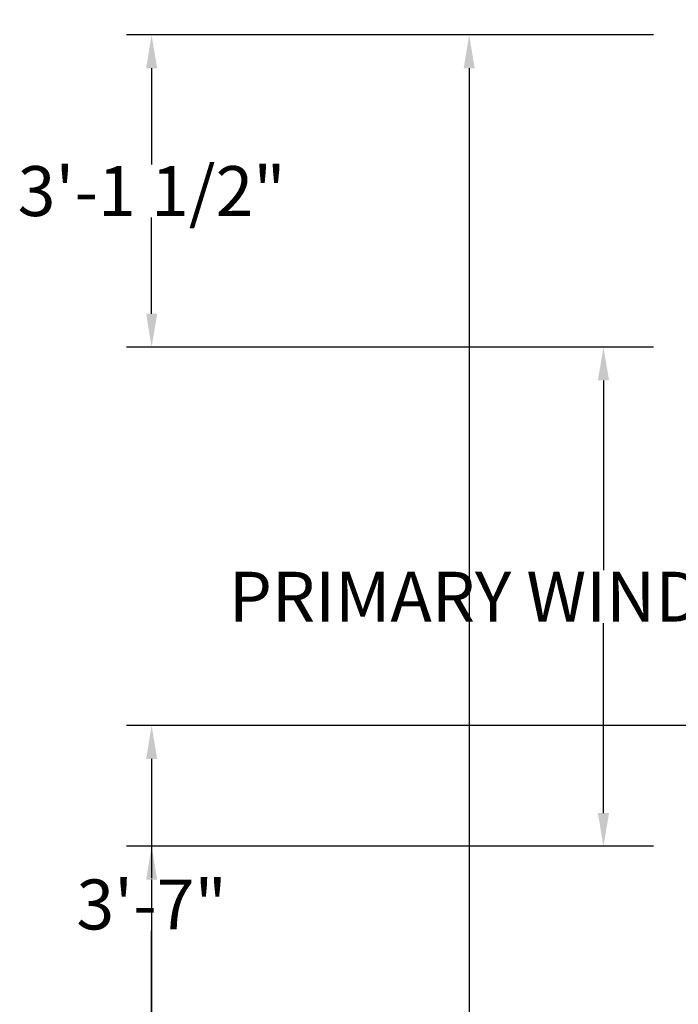
# Model space of a CAD drawing. Units: inches. Extents: x -59 to 502, y -260 to 136.
# Tile 2 of 8: x -54 to 25, y -53 to 66. Entities that reach past the tile are written whole.
import ezdxf

# ---------------------------------------------------------------- set-up
doc = ezdxf.new("R2010")
doc.units = ezdxf.units.IN
doc.header["$MEASUREMENT"] = 0
doc.layers.add('A-ANNO-DIMS', color=2, linetype='Continuous', lineweight=18)
doc.styles.get("Standard").update_dxf_attribs({"font": 'arial.ttf'})
doc.dimstyles.get("Standard").update_dxf_attribs({"dimtxt": 6, "dimasz": 4, "dimexe": 3, "dimexo": 3, "dimgap": 0.09, "dimtad": 0, "dimtih": 1, "dimtoh": 1, "dimdec": 1, "dimzin": 0, "dimdsep": 46, "dimlunit": 3, "dimtxsty": 'Standard', "dimcen": 0.09, "dimadec": 0, "dimazin": 0, "dimtfac": 1, "dimtdec": 1, "dimtofl": 0, "dimtmove": 0, "dimatfit": 3, "dimfxl": 1, "dimtolj": 1, "dimtzin": 0, "dimarcsym": 0})

# ---------------------------------------------------------------- blocks, each defined once
blk = doc.blocks.new('*D6')
at = {"layer": 'A-ANNO-DIMS', "color": 0, "lineweight": -2, "transparency": 16777216}
for p, q in [((22.46, 63.92), (-2.69, 63.92)), ((0.31, 59.92), (0.31, -58.98)), ((0.31, -184.08), (0.31, -65.18)), ((22.46, -188.08), (-2.69, -188.08))]:
    blk.add_line(p, q, dxfattribs=at)
at = {"layer": 'A-ANNO-DIMS', "color": 0, "transparency": 16777216}
for points in [[(-0.35, 59.92), (0.98, 59.92), (0.31, 63.92)], [(-0.35, -184.08), (0.98, -184.08), (0.31, -188.08)]]:
    blk.add_solid(points, dxfattribs=at)
at = {"layer": 'Defpoints', "color": 0, "transparency": 16777216}
for p in [(25.46, 63.92), (0.31, -188.08), (25.46, -188.08)]:
    blk.add_point(p, dxfattribs=at)
at = {"layer": 'A-ANNO-DIMS', "color": 0, "transparency": 16777216, "insert": (0.31, -62.08), "char_height": 6, "attachment_point": 5}
blk.add_mtext("\\A1;21'", dxfattribs=at)
blk = doc.blocks.new('*D41')
at = {"layer": 'A-ANNO-DIMS', "color": 0, "lineweight": -2, "transparency": 16777216}
for p, q in [((22.46, 26.41), (13.46, 26.41)), ((16.46, 22.41), (16.46, -0.4)), ((16.46, -29.59), (16.46, -6.79)), ((22.46, -33.59), (13.46, -33.59))]:
    blk.add_line(p, q, dxfattribs=at)
at = {"layer": 'A-ANNO-DIMS', "color": 0, "transparency": 16777216}
for points in [[(15.79, 22.41), (17.13, 22.41), (16.46, 26.41)], [(15.79, -29.59), (17.13, -29.59), (16.46, -33.59)]]:
    blk.add_solid(points, dxfattribs=at)
at = {"layer": 'Defpoints', "color": 0, "transparency": 16777216}
for p in [(25.46, 26.41), (16.46, -33.59), (25.46, -33.59)]:
    blk.add_point(p, dxfattribs=at)
at = {"layer": 'A-ANNO-DIMS', "color": 0, "transparency": 16777216, "insert": (16.46, -3.59), "char_height": 6, "attachment_point": 5}
blk.add_mtext('\\A1;PRIMARY WINDOW 5\'-0"', dxfattribs=at)
blk = doc.blocks.new('*D57')
at = {"layer": 'A-ANNO-DIMS', "color": 0, "lineweight": -2, "transparency": 16777216}
for p, q in [((25.46, 66.92), (25.46, 130.25)), ((184.38, 66.92), (184.38, 130.25)), ((29.46, 127.25), (94.81, 127.25)), ((180.38, 127.25), (115.03, 127.25))]:
    blk.add_line(p, q, dxfattribs=at)
at = {"layer": 'A-ANNO-DIMS', "color": 0, "transparency": 16777216}
for points in [[(29.46, 127.91), (29.46, 126.58), (25.46, 127.25)], [(180.38, 127.91), (180.38, 126.58), (184.38, 127.25)]]:
    blk.add_solid(points, dxfattribs=at)
at = {"layer": 'Defpoints', "color": 0, "transparency": 16777216}
for p in [(184.38, 127.25), (25.46, 63.92), (184.38, 63.92)]:
    blk.add_point(p, dxfattribs=at)
at = {"layer": 'A-ANNO-DIMS', "color": 0, "transparency": 16777216, "insert": (104.92, 127.25), "char_height": 6, "attachment_point": 5}
blk.add_mtext('\\A1;13\'-3"', dxfattribs=at)
blk = doc.blocks.new('*D59')
at = {"layer": 'A-ANNO-DIMS', "color": 0, "lineweight": -2, "transparency": 16777216}
for p, q in [((22.46, 63.92), (-40.87, 63.92)), ((-37.87, 59.92), (-37.87, 48.36)), ((-37.87, 30.41), (-37.87, 41.97)), ((22.46, 26.41), (-40.87, 26.41))]:
    blk.add_line(p, q, dxfattribs=at)
at = {"layer": 'A-ANNO-DIMS', "color": 0, "transparency": 16777216}
for points in [[(-38.53, 59.92), (-37.2, 59.92), (-37.87, 63.92)], [(-38.53, 30.41), (-37.2, 30.41), (-37.87, 26.41)]]:
    blk.add_solid(points, dxfattribs=at)
at = {"layer": 'Defpoints', "color": 0, "transparency": 16777216}
for p in [(25.46, 63.92), (-37.87, 26.41), (25.46, 26.41)]:
    blk.add_point(p, dxfattribs=at)
at = {"layer": 'A-ANNO-DIMS', "color": 0, "transparency": 16777216, "insert": (-37.87, 45.16), "char_height": 6, "attachment_point": 5}
blk.add_mtext('\\A1;3\'-1 1/2"', dxfattribs=at)
blk = doc.blocks.new('*D60')
at = {"layer": 'A-ANNO-DIMS', "color": 0, "lineweight": -2, "transparency": 16777216}
for p, q in [((22.46, -33.59), (-40.87, -33.59)), ((-37.87, -37.59), (-37.87, -70.44)), ((-37.87, -109.59), (-37.87, -76.75)), ((22.46, -113.59), (-40.87, -113.59))]:
    blk.add_line(p, q, dxfattribs=at)
at = {"layer": 'A-ANNO-DIMS', "color": 0, "transparency": 16777216}
for points in [[(-38.53, -37.59), (-37.2, -37.59), (-37.87, -33.59)], [(-38.53, -109.59), (-37.2, -109.59), (-37.87, -113.59)]]:
    blk.add_solid(points, dxfattribs=at)
at = {"layer": 'Defpoints', "color": 0, "transparency": 16777216}
for p in [(25.46, -33.59), (-37.87, -113.59), (25.46, -113.59)]:
    blk.add_point(p, dxfattribs=at)
at = {"layer": 'A-ANNO-DIMS', "color": 0, "transparency": 16777216, "insert": (-37.87, -73.59), "char_height": 6, "attachment_point": 5}
blk.add_mtext('\\A1;6\'-8"', dxfattribs=at)
blk = doc.blocks.new('*D68')
at = {"layer": 'A-ANNO-DIMS', "color": 0, "lineweight": -2, "transparency": 16777216}
for p, q in [((163.46, -19.08), (-40.87, -19.08)), ((-37.87, -23.08), (-37.87, -37.42)), ((-37.87, -58.08), (-37.87, -43.73)), ((163.46, -62.08), (-40.87, -62.08))]:
    blk.add_line(p, q, dxfattribs=at)
at = {"layer": 'A-ANNO-DIMS', "color": 0, "transparency": 16777216}
for points in [[(-38.53, -23.08), (-37.2, -23.08), (-37.87, -19.08)], [(-38.53, -58.08), (-37.2, -58.08), (-37.87, -62.08)]]:
    blk.add_solid(points, dxfattribs=at)
at = {"layer": 'Defpoints', "color": 0, "transparency": 16777216}
for p in [(166.46, -19.08), (-37.87, -62.08), (166.46, -62.08)]:
    blk.add_point(p, dxfattribs=at)
at = {"layer": 'A-ANNO-DIMS', "color": 0, "transparency": 16777216, "insert": (-37.87, -40.58), "char_height": 6, "attachment_point": 5}
blk.add_mtext('\\A1;3\'-7"', dxfattribs=at)

msp = doc.modelspace()

# ---------------------------------------------------------------- dimensions: what is measured, and where the dimension line sits
at = {"layer": 'A-ANNO-DIMS'}
dim = msp.add_linear_dim(base=(184.38, 127.25), p1=(25.46, 63.92), p2=(184.38, 63.92), dimstyle='Standard', override={"dimdec": 1, "dimlfac": 1, "dimrnd": 0, "dimzin": 1, "dimdsep": 46, "dimlunit": 4, "dimfrac": 2}, dxfattribs=at)
dim.commit()
dim.dimension.update_dxf_attribs({"geometry": '*D57', "text_midpoint": (104.92, 127.25)})
for base, p1, p2, override, picture, middle in [((-37.87, 26.41), (25.46, 63.92), (25.46, 26.41), {"dimdec": 1, "dimlfac": 1, "dimrnd": 0, "dimzin": 1, "dimdsep": 46, "dimlunit": 4, "dimfrac": 2}, '*D59', (-37.87, 45.16)), ((0.31, -188.08), (25.46, 63.92), (25.46, -188.08), {"dimclrd": 0, "dimclre": 0, "dimclrt": 0}, '*D6', (0.31, -62.08)), ((-37.87, -62.08), (166.46, -19.08), (166.46, -62.08), {"dimdec": 1, "dimlfac": 1, "dimrnd": 0, "dimzin": 1, "dimdsep": 46, "dimlunit": 4, "dimfrac": 2}, '*D68', (-37.87, -40.58)), ((-37.87, -113.59), (25.46, -33.59), (25.46, -113.59), {"dimdec": 1, "dimlfac": 1, "dimrnd": 0, "dimzin": 1, "dimdsep": 46, "dimlunit": 4, "dimfrac": 2}, '*D60', (-37.87, -73.59))]:
    dim = msp.add_linear_dim(base=base, p1=p1, p2=p2, angle=90, dimstyle='Standard', override=override, dxfattribs=at)
    dim.commit()
    dim.dimension.update_dxf_attribs({"geometry": picture, "text_midpoint": middle})
dim = msp.add_linear_dim(base=(16.46, -33.59), p1=(25.46, 26.41), p2=(25.46, -33.59), angle=270, text='PRIMARY WINDOW <>', dimstyle='Standard', override={"dimdec": 1, "dimlfac": 1, "dimrnd": 0, "dimzin": 1, "dimdsep": 46, "dimlunit": 4, "dimfrac": 2}, dxfattribs=at)
dim.commit()
dim.dimension.update_dxf_attribs({"geometry": '*D41', "text_midpoint": (16.46, -3.59)})

doc.saveas('drawing.dxf')
